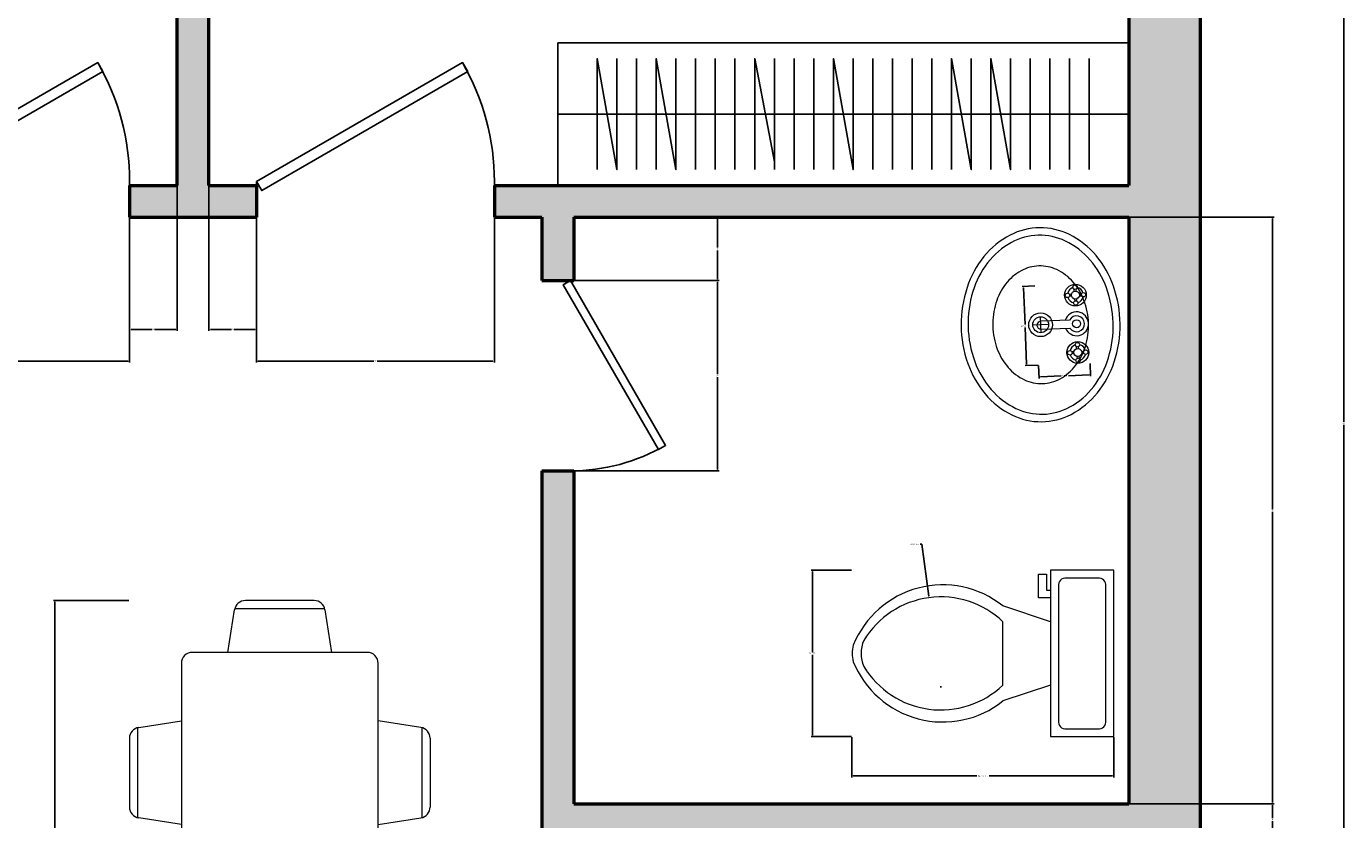
# Model space of a CAD drawing. Units: inches. Extents: x 2130 to 2425, y 2862 to 3216.
# Tile 3 of 4: x 2259 to 2425, y 2989 to 3089. Entities that reach past the tile are written whole.
import ezdxf

# ---------------------------------------------------------------- set-up
doc = ezdxf.new("R2010")
doc.units = ezdxf.units.IN
for name, color, linetype, lineweight in [('A-ANNO-DIMS', 2, 'Continuous', 18), ('A-DOOR', 3, 'Continuous', 25), ('A-FLOR-CASE', 9, 'Continuous', 25), ('A-FLOR-FIXT', 9, 'Continuous', 18), ('A-FURN', 8, 'Continuous', 18), ('A-WALL', 7, 'Continuous', 50), ('A-WALL-PATT', 18, 'Continuous', 13)]:
    doc.layers.add(name, color=color, linetype=linetype, lineweight=lineweight)
doc.styles.get("Standard").update_dxf_attribs({"font": 'arial.ttf'})
doc.dimstyles.get("Standard").update_dxf_attribs({"dimtxt": 0.18, "dimasz": 0.18, "dimexe": 0.18, "dimexo": 0.0625, "dimgap": 0.09, "dimtad": 0, "dimtih": 1, "dimtoh": 1, "dimdec": 4, "dimzin": 0, "dimdsep": 46, "dimtxsty": 'Standard', "dimcen": 0.09, "dimadec": 0, "dimazin": 0, "dimtfac": 1, "dimtdec": 4, "dimtofl": 0, "dimtmove": 0, "dimatfit": 3, "dimfxl": 1, "dimtolj": 1, "dimtzin": 0, "dimarcsym": 0})

# ---------------------------------------------------------------- blocks, each defined once
blk = doc.blocks.new('Toilet - top')
for p, q in [((9.5, -6), (9.5, -2)), ((-8, -8.5), (-8, -8)), ((-7, -8), (-7, -9.5)), ((-4, -8), (-6, -14)), ((4, -8), (6, -14)), ((-10, -8.5), (-8, -8.5)), ((-10, -9.5), (-10, -8.5)), ((-7, -9.5), (-10, -9.5)), ((4, -14), (-4, -14))]:
    blk.add_line(p, q)
blk.add_lwpolyline([(10.5, -8), (10.5, 0), (-10.5, 0), (-10.5, -8)], close=True)
for points in [[(8.5, -1), (-8.5, -1)], [(-9.5, -2), (-9.5, -6)], [(-8.5, -7), (8.5, -7)]]:
    blk.add_lwpolyline(points)
for centre, radius, start, end in [((-8.62, -1.88), 0.884, 81.8699, 188.1301), ((8.62, -1.88), 0.884, 351.8699, 98.1301), ((-8.62, -6.12), 0.884, 171.8699, 278.1301), ((8.62, -6.12), 0.884, 261.8699, 8.1301), ((3.52, -21.58), 12.17, 141.4691, 247.9714), ((4.2, -21.82), 11.33, 136.3677, 238.9468), ((-3.52, -21.58), 12.17, 292.0284, 38.5307), ((-4.2, -21.82), 11.33, 301.053, 43.6321), ((0, -27.88), 4, 245.7318, 294.2682), ((0, -29), 4, 254.8605, 285.1395)]:
    blk.add_arc(centre, radius, start, end)
blk = doc.blocks.new('Dining Set - 36 x 72 in.')
for p, q in [((-20.29, 27.5), (-7.71, 27.5)), ((7.71, 27.5), (20.29, 27.5)), ((-22.26, 25.81), (-23.48, 18)), ((-22.23, 26), (-5.76, 26)), ((-4.52, 18), (-5.74, 25.81)), ((5.74, 25.81), (4.52, 18)), ((5.77, 26), (22.24, 26)), ((23.48, 18), (22.26, 25.81)), ((34, 18), (-34, 18)), ((-36, 16), (-36, -16)), ((36, -16), (36, 16)), ((-44, 8.23), (-44, -8.24)), ((-43.81, 8.26), (-36, 9.48)), ((43.81, 8.26), (36, 9.48)), ((44, 8.23), (44, -8.24)), ((-45.5, 6.29), (-45.5, -6.29)), ((45.5, 6.29), (45.5, -6.29)), ((-36, -9.48), (-43.81, -8.26)), ((36, -9.48), (43.81, -8.26)), ((-34, -18), (34, -18)), ((-22.26, -25.81), (-23.48, -18)), ((-4.52, -18), (-5.74, -25.81)), ((5.74, -25.81), (4.52, -18)), ((23.48, -18), (22.26, -25.81)), ((-22.23, -26), (-5.76, -26)), ((5.77, -26), (22.24, -26)), ((-20.29, -27.5), (-7.71, -27.5)), ((7.71, -27.5), (20.29, -27.5))]:
    blk.add_line(p, q)
for centre, start, end in [((-20.29, 25.5), 90, 171.1198), ((-7.71, 25.5), 8.881, 90), ((7.71, 25.5), 90, 171.1198), ((20.29, 25.5), 8.881, 90), ((-34, 16), 90, 180), ((34, 16), 0, 90), ((-43.5, 6.29), 98.8806, 180), ((43.5, 6.29), 0, 81.1194), ((-43.5, -6.29), 180, 261.1194), ((43.5, -6.29), 278.8806, 0), ((-34, -16), 180, 270), ((34, -16), 270, 0), ((-20.29, -25.5), 188.8802, 270), ((-7.71, -25.5), 270, 351.1191), ((7.71, -25.5), 188.8802, 270), ((20.29, -25.5), 270, 351.1191)]:
    blk.add_arc(centre, 2, start, end)
blk = doc.blocks.new('Sink - Oval top')
for p, q in [((-1, 0), (1, 0)), ((0, 1), (0, -1))]:
    blk.add_line(p, q)
for points in [[(-12.23, 0.39, 0.117634), (-11.46, -3.36, 0.104469), (-8.88, -6.8, 0.090016), (-5.08, -9.07, 0.08192), (-0.32, -10.02, 0.08192), (4.49, -9.38, 0.090016), (8.42, -7.36, 0.104469), (11.22, -4.09, 0.117634), (12.23, -0.39, 0.117634), (11.46, 3.36, 0.104469), (8.88, 6.8, 0.090016), (5.08, 9.07, 0.08192), (0.32, 10.02, 0.08192), (-4.49, 9.38, 0.090016), (-8.42, 7.36, 0.104469), (-11.22, 4.09, 0.117634)], [(-11.29, 0.16, 0.118622), (-10.52, -3.25, 0.104678), (-8.07, -6.36, 0.089562), (-4.54, -8.37, 0.081185), (-0.13, -9.15, 0.081185), (4.3, -8.49, 0.089562), (7.89, -6.58, 0.104678), (10.42, -3.55, 0.118622), (11.29, -0.16, 0.118622), (10.52, 3.25, 0.104678), (8.07, 6.36, 0.089562), (4.54, 8.37, 0.081185), (0.13, 9.15, 0.081185), (-4.3, 8.49, 0.089562), (-7.89, 6.58, 0.104678), (-10.42, 3.55, 0.118622)], [(-7.42, 0.08, 0.118283), (-6.91, -2.17, 0.104607), (-5.29, -4.21, 0.089718), (-2.97, -5.53, 0.081436), (-0.07, -6.04, 0.081436), (2.84, -5.59, 0.089718), (5.2, -4.33, 0.104607), (6.86, -2.32, 0.118283), (7.42, -0.08, 0.118283), (6.91, 2.17, 0.104607), (5.29, 4.21, 0.089718), (2.97, 5.53, 0.081436), (0.07, 6.04, 0.081436), (-2.84, 5.59, 0.089718), (-5.2, 4.33, 0.104607), (-6.86, 2.32, 0.118283)]]:
    blk.add_lwpolyline(points, format="xyb", close=True)
for radius in [1.5, 1]:
    blk.add_circle((0, 0), radius)
blk = doc.blocks.new('Faucet - Bathroom top')
for p, q in [((-4.107, 0.125), (-4.375, 0.125)), ((-3.75, 0.4788), (-3.75, 0.75)), ((-3.5, 0.482), (-3.5, 0.75)), ((-3.1461, 0.125), (-2.875, 0.125)), ((3.143, 0.125), (2.875, 0.125)), ((3.5, 0.4788), (3.5, 0.75)), ((3.75, 0.482), (3.75, 0.75)), ((4.1039, 0.125), (4.375, 0.125)), ((-4.1039, -0.125), (-4.375, -0.125)), ((-3.75, -0.4821), (-3.75, -0.75)), ((-3.5, -0.4789), (-3.5, -0.75)), ((-3.143, -0.125), (-2.875, -0.125)), ((-0.5, -0.8639), (-0.5, -4.5)), ((0.5, -4.5), (0.5, -0.8631)), ((3.1461, -0.125), (2.875, -0.125)), ((3.5, -0.4821), (3.5, -0.75)), ((3.75, -0.4789), (3.75, -0.75)), ((4.107, -0.125), (4.375, -0.125))]:
    blk.add_line(p, q)
for centre, radius in [((-3.625, 0), 1.375), ((-4.625, 0), 0.2795), ((-3.625, 0), 0.5), ((-3.625, 1), 0.2795), ((-2.625, 0), 0.2795), ((0, 0), 0.5), ((3.625, 0), 1.375), ((2.625, 0), 0.2795), ((3.625, 0), 0.5), ((3.625, 1), 0.2795), ((4.625, 0), 0.2795), ((-3.625, -1), 0.2795), ((3.625, -1), 0.2795)]:
    blk.add_circle(centre, radius)
for centre, radius, start, end in [((-3.625, 0), 1, 105.2407, 164.2093), ((-3.625, 0), 1, 16.44125, 74.07887), ((0, 0), 1.5, 289.6514, 250.3603), ((0, 0), 1, 300.3431, 239.7554), ((3.625, 0), 1, 106.12, 164.0884), ((3.625, 0), 1, 16.23422, 73.90469), ((-3.625, 0), 1, 196.2342, 253.9047), ((-3.625, 0), 1, 286.12, 344.0884), ((3.625, 0), 1, 196.4413, 254.0789), ((3.625, 0), 1, 285.2407, 344.2093), ((0, -4.5), 0.5, 180, 0)]:
    blk.add_arc(centre, radius, start, end)
blk = doc.blocks.new('*U10')
for p, q in [((0, 0), (0, -6)), ((40, 0), (40, -6))]:
    blk.add_line(p, q)
blk.add_lwpolyline([(0, 0), (34.64, 20), (35.52, 18.48), (0.87, -1.52)], close=True)
blk.add_arc((0, 0), 40, 0, 30)
blk = doc.blocks.new('WARDROBE-72X18IN')
for p, q in [((0, 0), (0, 72)), ((0, 72), (18, 72)), ((9, 72), (9, 0)), ((18, 72), (18, 0)), ((2, 62.07), (16, 62.07)), ((2, 54.62), (16, 54.62)), ((2, 52.14), (16, 52.14)), ((2, 49.66), (16, 49.66)), ((2, 44.69), (16, 44.69)), ((2, 42.21), (16, 42.21)), ((2, 39.72), (16, 39.72)), ((2, 32.28), (16, 32.28)), ((2, 29.79), (16, 29.79)), ((2, 27.31), (16, 27.31)), ((2, 24.83), (16, 24.83)), ((2, 12.41), (16, 12.41)), ((2, 9.93), (16, 9.93)), ((2, 7.45), (16, 7.45)), ((2, 4.97), (16, 4.97)), ((18, 0), (0, 0))]:
    blk.add_line(p, q)
for points in [[(2, 67.03), (16, 67.03), (2, 64.55), (16, 64.55)], [(2, 59.59), (16, 59.59), (2, 57.1), (16, 57.1)], [(2, 47.17), (16, 47.17), (2.98, 44.69)], [(2, 37.24), (16, 37.24), (2, 34.76), (16, 34.76)], [(2, 22.35), (16, 22.35), (2, 19.86), (16, 19.86)], [(2, 17.38), (16, 17.38), (2, 14.9), (16, 14.9)]]:
    blk.add_lwpolyline(points)
blk.add_lwpolyline([(0, 0), (18, 0)], close=True)
blk = doc.blocks.new('*D21')
at = {"layer": 'A-ANNO-DIMS', "color": 0, "lineweight": -2, "transparency": 16777216}
for p, q in [((2362.63, 2999.36), (2362.63, 2994.28)), ((2395.68, 2999.36), (2395.68, 2994.28)), ((2362.81, 2994.46), (2378.38, 2994.46)), ((2395.5, 2994.46), (2379.93, 2994.46))]:
    blk.add_line(p, q, dxfattribs=at)
at = {"layer": 'A-ANNO-DIMS', "color": 0, "transparency": 16777216}
for points in [[(2362.81, 2994.49), (2362.81, 2994.43), (2362.63, 2994.46)], [(2395.5, 2994.49), (2395.5, 2994.43), (2395.68, 2994.46)]]:
    blk.add_solid(points, dxfattribs=at)
at = {"layer": 'Defpoints', "color": 0, "transparency": 16777216}
for p in [(2362.63, 2999.42), (2395.68, 2999.42), (2395.68, 2994.46)]:
    blk.add_point(p, dxfattribs=at)
at = {"layer": 'A-ANNO-DIMS', "color": 0, "transparency": 16777216, "insert": (2379.15, 2994.46), "char_height": 0.18, "attachment_point": 5}
blk.add_mtext('\\A1;WC 33 TYP.', dxfattribs=at)
blk = doc.blocks.new('*D22')
at = {"layer": 'A-ANNO-DIMS', "color": 0, "lineweight": -2, "transparency": 16777216}
for p, q in [((2362.57, 3020.42), (2357.49, 3020.42)), ((2357.67, 3020.24), (2357.67, 3010.1)), ((2357.67, 2999.6), (2357.67, 3009.74)), ((2362.57, 2999.42), (2357.49, 2999.42))]:
    blk.add_line(p, q, dxfattribs=at)
at = {"layer": 'A-ANNO-DIMS', "color": 0, "transparency": 16777216}
for points in [[(2357.64, 3020.24), (2357.7, 3020.24), (2357.67, 3020.42)], [(2357.64, 2999.6), (2357.7, 2999.6), (2357.67, 2999.42)]]:
    blk.add_solid(points, dxfattribs=at)
at = {"layer": 'Defpoints', "color": 0, "transparency": 16777216}
for p in [(2362.63, 3020.42), (2357.67, 2999.42), (2362.63, 2999.42)]:
    blk.add_point(p, dxfattribs=at)
at = {"layer": 'A-ANNO-DIMS', "color": 0, "transparency": 16777216, "insert": (2357.67, 3009.92), "char_height": 0.18, "attachment_point": 5}
blk.add_mtext('\\A1;21 TYP.', dxfattribs=at)
blk = doc.blocks.new('*D25')
at = {"layer": 'A-ANNO-DIMS', "color": 0, "lineweight": -2, "transparency": 16777216}
for p, q in [((2385.71, 3056.29), (2384.1, 3056.22)), ((2384.28, 3056.05), (2384.48, 3051.42)), ((2384.68, 3046.42), (2384.49, 3051.05)), ((2386.13, 3046.3), (2384.51, 3046.23))]:
    blk.add_line(p, q, dxfattribs=at)
at = {"layer": 'A-ANNO-DIMS', "color": 0, "transparency": 16777216}
for points in [[(2384.31, 3056.05), (2384.25, 3056.05), (2384.28, 3056.23)], [(2384.71, 3046.42), (2384.65, 3046.42), (2384.69, 3046.24)]]:
    blk.add_solid(points, dxfattribs=at)
at = {"layer": 'Defpoints', "color": 0, "transparency": 16777216}
for p in [(2385.78, 3056.29), (2384.69, 3046.24), (2386.19, 3046.3)]:
    blk.add_point(p, dxfattribs=at)
at = {"layer": 'A-ANNO-DIMS', "color": 0, "transparency": 16777216, "insert": (2384.48, 3051.24), "char_height": 0.18, "attachment_point": 5}
blk.add_mtext('\\A1;TAP 10 TYP.', dxfattribs=at)
blk = doc.blocks.new('*D26')
at = {"layer": 'A-ANNO-DIMS', "color": 0, "lineweight": -2, "transparency": 16777216}
for p, q in [((2392.69, 3046.51), (2392.75, 3044.89)), ((2386.19, 3046.24), (2386.26, 3044.62)), ((2386.43, 3044.81), (2389.04, 3044.92)), ((2392.57, 3045.07), (2389.96, 3044.96))]:
    blk.add_line(p, q, dxfattribs=at)
at = {"layer": 'A-ANNO-DIMS', "color": 0, "transparency": 16777216}
for points in [[(2386.43, 3044.84), (2386.43, 3044.78), (2386.25, 3044.8)], [(2392.57, 3045.1), (2392.57, 3045.04), (2392.75, 3045.07)]]:
    blk.add_solid(points, dxfattribs=at)
at = {"layer": 'Defpoints', "color": 0, "transparency": 16777216}
for p in [(2392.68, 3046.57), (2386.19, 3046.3), (2392.75, 3045.07)]:
    blk.add_point(p, dxfattribs=at)
at = {"layer": 'A-ANNO-DIMS', "color": 0, "transparency": 16777216, "insert": (2389.5, 3044.94), "char_height": 0.18, "attachment_point": 5}
blk.add_mtext('\\A1;7 TYP.', dxfattribs=at)
blk = doc.blocks.new('*D29')
at = {"layer": 'A-ANNO-DIMS', "color": 0, "lineweight": -2, "transparency": 16777216}
for p, q in [((2271.46, 3016.6), (2261.94, 3016.6)), ((2262.12, 3016.42), (2262.12, 2985.41)), ((2262.12, 2954.04), (2262.12, 2985.05)), ((2271.46, 2953.86), (2261.94, 2953.86))]:
    blk.add_line(p, q, dxfattribs=at)
at = {"layer": 'A-ANNO-DIMS', "color": 0, "transparency": 16777216}
for points in [[(2262.09, 3016.42), (2262.15, 3016.42), (2262.12, 3016.6)], [(2262.09, 2954.04), (2262.15, 2954.04), (2262.12, 2953.86)]]:
    blk.add_solid(points, dxfattribs=at)
at = {"layer": 'Defpoints', "color": 0, "transparency": 16777216}
for p in [(2271.53, 3016.6), (2262.12, 2953.86), (2271.53, 2953.86)]:
    blk.add_point(p, dxfattribs=at)
at = {"layer": 'A-ANNO-DIMS', "color": 0, "transparency": 16777216, "insert": (2262.12, 2985.23), "char_height": 0.18, "attachment_point": 5}
blk.add_mtext('\\A1;DINING SET 63', dxfattribs=at)
blk = doc.blocks.new('*D36')
at = {"layer": 'A-ANNO-DIMS', "color": 0, "lineweight": -2, "transparency": 16777216}
for p, q in [((2406.61, 3197.95), (2424.88, 3197.95)), ((2424.7, 3197.77), (2424.7, 3039.14)), ((2424.7, 2880.13), (2424.7, 3038.77)), ((2406.61, 2879.95), (2424.88, 2879.95))]:
    blk.add_line(p, q, dxfattribs=at)
at = {"layer": 'A-ANNO-DIMS', "color": 0, "transparency": 16777216}
for points in [[(2424.67, 3197.77), (2424.73, 3197.77), (2424.7, 3197.95)], [(2424.67, 2880.13), (2424.73, 2880.13), (2424.7, 2879.95)]]:
    blk.add_solid(points, dxfattribs=at)
at = {"layer": 'Defpoints', "color": 0, "transparency": 16777216}
for p in [(2406.55, 3197.95), (2424.7, 3197.95), (2406.55, 2879.95)]:
    blk.add_point(p, dxfattribs=at)
at = {"layer": 'A-ANNO-DIMS', "color": 0, "transparency": 16777216, "insert": (2424.7, 3038.95), "char_height": 0.18, "attachment_point": 5}
blk.add_mtext('\\A1;318', dxfattribs=at)
blk = doc.blocks.new('*D54')
at = {"layer": 'A-ANNO-DIMS', "color": 0, "lineweight": -2, "transparency": 16777216}
for p, q in [((2397.612727, 3064.954394), (2415.880227, 3064.954394)), ((2415.700227, 3064.774394), (2415.700227, 3028.134394)), ((2415.700227, 2991.134394), (2415.700227, 3027.774394)), ((2397.612727, 2990.954394), (2415.880227, 2990.954394))]:
    blk.add_line(p, q, dxfattribs=at)
at = {"layer": 'A-ANNO-DIMS', "color": 0, "transparency": 16777216}
for points in [[(2415.670227, 3064.774394), (2415.730227, 3064.774394), (2415.700227, 3064.954394)], [(2415.670227, 2991.134394), (2415.730227, 2991.134394), (2415.700227, 2990.954394)]]:
    blk.add_solid(points, dxfattribs=at)
at = {"layer": 'Defpoints', "color": 0, "transparency": 16777216}
for p in [(2397.550227, 3064.954394), (2397.550227, 2990.954394), (2415.700227, 2990.954394)]:
    blk.add_point(p, dxfattribs=at)
at = {"layer": 'A-ANNO-DIMS', "color": 0, "transparency": 16777216, "insert": (2415.700227, 3027.954394), "char_height": 0.18, "attachment_point": 5}
blk.add_mtext('\\A1;74', dxfattribs=at)
blk = doc.blocks.new('*D55')
at = {"layer": 'A-ANNO-DIMS', "color": 0, "lineweight": -2, "transparency": 16777216}
for p, q in [((2397.612727, 2990.954394), (2415.880227, 2990.954394)), ((2415.700227, 2990.774394), (2415.700227, 2989.134394)), ((2415.700227, 2987.134394), (2415.700227, 2988.774394)), ((2397.612727, 2986.954394), (2415.880227, 2986.954394))]:
    blk.add_line(p, q, dxfattribs=at)
at = {"layer": 'A-ANNO-DIMS', "color": 0, "transparency": 16777216}
for points in [[(2415.670227, 2990.774394), (2415.730227, 2990.774394), (2415.700227, 2990.954394)], [(2415.670227, 2987.134394), (2415.730227, 2987.134394), (2415.700227, 2986.954394)]]:
    blk.add_solid(points, dxfattribs=at)
at = {"layer": 'Defpoints', "color": 0, "transparency": 16777216}
for p in [(2397.550227, 2990.954394), (2397.550227, 2986.954394), (2415.700227, 2986.954394)]:
    blk.add_point(p, dxfattribs=at)
at = {"layer": 'A-ANNO-DIMS', "color": 0, "transparency": 16777216, "insert": (2415.700227, 2988.954394), "char_height": 0.18, "attachment_point": 5}
blk.add_mtext('\\A1;4', dxfattribs=at)
blk = doc.blocks.new('*D57')
at = {"layer": 'A-ANNO-DIMS', "color": 0, "lineweight": -2, "transparency": 16777216}
for p, q in [((2241.55, 3064.89), (2241.55, 3046.62)), ((2271.55, 3064.89), (2271.55, 3046.62)), ((2241.73, 3046.8), (2256.33, 3046.8)), ((2271.37, 3046.8), (2256.77, 3046.8))]:
    blk.add_line(p, q, dxfattribs=at)
at = {"layer": 'A-ANNO-DIMS', "color": 0, "transparency": 16777216}
for points in [[(2241.73, 3046.83), (2241.73, 3046.77), (2241.55, 3046.8)], [(2271.37, 3046.83), (2271.37, 3046.77), (2271.55, 3046.8)]]:
    blk.add_solid(points, dxfattribs=at)
at = {"layer": 'Defpoints', "color": 0, "transparency": 16777216}
for p in [(2241.55, 3064.95), (2271.55, 3064.95), (2241.55, 3046.8)]:
    blk.add_point(p, dxfattribs=at)
at = {"layer": 'A-ANNO-DIMS', "color": 0, "transparency": 16777216, "insert": (2256.55, 3046.8), "char_height": 0.18, "attachment_point": 5}
blk.add_mtext('\\A1;30', dxfattribs=at)
blk = doc.blocks.new('*D58')
at = {"layer": 'A-ANNO-DIMS', "color": 0, "lineweight": -2, "transparency": 16777216}
for p, q in [((2271.55, 3068.89), (2271.55, 3050.62)), ((2277.55, 3068.89), (2277.55, 3050.62)), ((2271.73, 3050.8), (2274.4, 3050.8)), ((2277.37, 3050.8), (2274.7, 3050.8))]:
    blk.add_line(p, q, dxfattribs=at)
at = {"layer": 'A-ANNO-DIMS', "color": 0, "transparency": 16777216}
for points in [[(2271.73, 3050.83), (2271.73, 3050.77), (2271.55, 3050.8)], [(2277.37, 3050.83), (2277.37, 3050.77), (2277.55, 3050.8)]]:
    blk.add_solid(points, dxfattribs=at)
at = {"layer": 'Defpoints', "color": 0, "transparency": 16777216}
for p in [(2271.55, 3068.95), (2277.55, 3068.95), (2271.55, 3050.8)]:
    blk.add_point(p, dxfattribs=at)
at = {"layer": 'A-ANNO-DIMS', "color": 0, "transparency": 16777216, "insert": (2274.55, 3050.8), "char_height": 0.18, "attachment_point": 5}
blk.add_mtext('\\A1;6', dxfattribs=at)
blk = doc.blocks.new('*D59')
at = {"layer": 'A-ANNO-DIMS', "color": 0, "lineweight": -2, "transparency": 16777216}
for p, q in [((2281.55, 3068.89), (2281.55, 3050.62)), ((2287.55, 3068.89), (2287.55, 3050.62)), ((2281.73, 3050.8), (2284.4, 3050.8)), ((2287.37, 3050.8), (2284.7, 3050.8))]:
    blk.add_line(p, q, dxfattribs=at)
at = {"layer": 'A-ANNO-DIMS', "color": 0, "transparency": 16777216}
for points in [[(2281.73, 3050.83), (2281.73, 3050.77), (2281.55, 3050.8)], [(2287.37, 3050.83), (2287.37, 3050.77), (2287.55, 3050.8)]]:
    blk.add_solid(points, dxfattribs=at)
at = {"layer": 'Defpoints', "color": 0, "transparency": 16777216}
for p in [(2281.55, 3068.95), (2287.55, 3068.95), (2281.55, 3050.8)]:
    blk.add_point(p, dxfattribs=at)
at = {"layer": 'A-ANNO-DIMS', "color": 0, "transparency": 16777216, "insert": (2284.55, 3050.8), "char_height": 0.18, "attachment_point": 5}
blk.add_mtext('\\A1;6', dxfattribs=at)
blk = doc.blocks.new('*D60')
at = {"layer": 'A-ANNO-DIMS', "color": 0, "lineweight": -2, "transparency": 16777216}
for p, q in [((2287.55, 3064.89), (2287.55, 3046.62)), ((2317.55, 3064.89), (2317.55, 3046.62)), ((2287.73, 3046.8), (2302.33, 3046.8)), ((2317.37, 3046.8), (2302.77, 3046.8))]:
    blk.add_line(p, q, dxfattribs=at)
at = {"layer": 'A-ANNO-DIMS', "color": 0, "transparency": 16777216}
for points in [[(2287.73, 3046.83), (2287.73, 3046.77), (2287.55, 3046.8)], [(2317.37, 3046.83), (2317.37, 3046.77), (2317.55, 3046.8)]]:
    blk.add_solid(points, dxfattribs=at)
at = {"layer": 'Defpoints', "color": 0, "transparency": 16777216}
for p in [(2287.55, 3064.95), (2317.55, 3064.95), (2287.55, 3046.8)]:
    blk.add_point(p, dxfattribs=at)
at = {"layer": 'A-ANNO-DIMS', "color": 0, "transparency": 16777216, "insert": (2302.55, 3046.8), "char_height": 0.18, "attachment_point": 5}
blk.add_mtext('\\A1;30', dxfattribs=at)
blk = doc.blocks.new('*D63')
at = {"layer": 'A-ANNO-DIMS', "color": 0, "lineweight": -2, "transparency": 16777216}
for p, q in [((2327.61, 3056.95), (2345.88, 3056.95)), ((2345.7, 3056.77), (2345.7, 3045.13)), ((2345.7, 3033.13), (2345.7, 3044.77)), ((2327.61, 3032.95), (2345.88, 3032.95))]:
    blk.add_line(p, q, dxfattribs=at)
at = {"layer": 'A-ANNO-DIMS', "color": 0, "transparency": 16777216}
for points in [[(2345.67, 3056.77), (2345.73, 3056.77), (2345.7, 3056.95)], [(2345.67, 3033.13), (2345.73, 3033.13), (2345.7, 3032.95)]]:
    blk.add_solid(points, dxfattribs=at)
at = {"layer": 'Defpoints', "color": 0, "transparency": 16777216}
for p in [(2327.55, 3056.95), (2327.55, 3032.95), (2345.7, 3032.95)]:
    blk.add_point(p, dxfattribs=at)
at = {"layer": 'A-ANNO-DIMS', "color": 0, "transparency": 16777216, "insert": (2345.7, 3044.95), "char_height": 0.18, "attachment_point": 5}
blk.add_mtext('\\A1;24', dxfattribs=at)
blk = doc.blocks.new('*D64')
at = {"layer": 'A-ANNO-DIMS', "color": 0, "lineweight": -2, "transparency": 16777216}
for p, q in [((2327.61, 3064.95), (2345.88, 3064.95)), ((2345.7, 3064.77), (2345.7, 3061.14)), ((2345.7, 3057.13), (2345.7, 3060.77)), ((2327.61, 3056.95), (2345.88, 3056.95))]:
    blk.add_line(p, q, dxfattribs=at)
at = {"layer": 'A-ANNO-DIMS', "color": 0, "transparency": 16777216}
for points in [[(2345.67, 3064.77), (2345.73, 3064.77), (2345.7, 3064.95)], [(2345.67, 3057.13), (2345.73, 3057.13), (2345.7, 3056.95)]]:
    blk.add_solid(points, dxfattribs=at)
at = {"layer": 'Defpoints', "color": 0, "transparency": 16777216}
for p in [(2327.55, 3064.95), (2327.55, 3056.95), (2345.7, 3056.95)]:
    blk.add_point(p, dxfattribs=at)
at = {"layer": 'A-ANNO-DIMS', "color": 0, "transparency": 16777216, "insert": (2345.7, 3060.95), "char_height": 0.18, "attachment_point": 5}
blk.add_mtext('\\A1;8', dxfattribs=at)
blk = doc.blocks.new('*D75')
at = {"layer": 'A-ANNO-DIMS', "color": 0, "lineweight": -2, "transparency": 16777216}
for p, q in [((2371.26, 3023.69), (2371.44, 3023.69)), ((2371.44, 3023.69), (2372.33, 3017.13)), ((2373.77, 3005.72), (2373.95, 3005.72)), ((2373.86, 3005.63), (2373.86, 3005.81))]:
    blk.add_line(p, q, dxfattribs=at)
at = {"layer": 'A-ANNO-DIMS', "color": 0, "transparency": 16777216}
blk.add_solid([(2372.36, 3017.13), (2372.3, 3017.12), (2372.35, 3016.95)], dxfattribs=at)
at = {"layer": 'Defpoints', "color": 0, "transparency": 16777216}
for p in [(2372.35, 3016.95), (2373.86, 3005.72)]:
    blk.add_point(p, dxfattribs=at)
at = {"layer": 'A-ANNO-DIMS', "color": 0, "transparency": 16777216, "insert": (2370.59, 3023.69), "char_height": 0.18, "attachment_point": 5}
blk.add_mtext('\\A1;4X R11.33', dxfattribs=at)

msp = doc.modelspace()

# ---------------------------------------------------------------- hatches: boundary and pattern name
at = {"layer": 'A-WALL-PATT'}
h = msp.add_hatch(color=256, dxfattribs=at)
h.dxf.hatch_style = 1
h.paths.add_polyline_path([(2319.6433, 3197.9544), (2234.3228, 3197.9544), (2234.3228, 3188.9544), (2277.5502, 3188.9544), (2277.5502, 3116.9544), (2277.5502, 3068.9544), (2271.5502, 3068.9544), (2271.5502, 3064.9544), (2281.5502, 3064.9544), (2287.5502, 3064.9544), (2287.5502, 3068.9544), (2281.5502, 3068.9544), (2281.5502, 3188.9544), (2319.6433, 3188.9544)])
h = msp.add_hatch(color=256, dxfattribs=at)
h.dxf.hatch_style = 1
h.paths.add_polyline_path([(2406.5502, 3197.9544), (2367.6433, 3197.9544), (2367.6433, 3188.9544), (2397.5502, 3188.9544), (2397.5502, 3068.9544), (2325.5502, 3068.9544), (2317.5502, 3068.9544), (2317.5502, 3064.9544), (2323.5502, 3064.9544), (2323.5502, 3056.9544), (2327.5502, 3056.9544), (2327.5502, 3064.9544), (2397.5502, 3064.9544), (2397.5502, 2990.9544), (2327.5502, 2990.9544), (2327.5502, 3032.9544), (2323.5502, 3032.9544), (2323.5502, 2986.9544), (2323.5502, 2961.9544), (2327.5502, 2961.9544), (2327.5502, 2986.9544), (2397.5502, 2986.9544), (2397.5502, 2966.8556), (2406.5502, 2966.8556)])

# ---------------------------------------------------------------- linework, layer by layer
at = {"layer": 'A-WALL'}
for p, q in [((2277.5502, 3068.9544), (2277.5502, 3188.9544)), ((2281.5502, 3068.9544), (2281.5502, 3188.9544)), ((2397.5502, 3188.9544), (2397.5502, 3068.9544)), ((2271.5502, 3068.9544), (2271.5502, 3064.9544)), ((2271.5502, 3068.9544), (2277.5502, 3068.9544)), ((2281.5502, 3068.9544), (2287.5502, 3068.9544)), ((2287.5502, 3068.9544), (2287.5502, 3064.9544)), ((2317.5502, 3068.9544), (2317.5502, 3064.9544)), ((2317.5502, 3068.9544), (2397.5502, 3068.9544)), ((2271.5502, 3064.9544), (2281.5502, 3064.9544)), ((2281.5502, 3064.9544), (2287.5502, 3064.9544)), ((2317.5502, 3064.9544), (2323.5502, 3064.9544)), ((2323.5502, 3064.9544), (2323.5502, 3056.9544)), ((2327.5502, 3064.9544), (2327.5502, 3056.9544)), ((2327.5502, 3064.9544), (2397.5502, 3064.9544)), ((2397.5502, 3064.9544), (2397.5502, 2990.9544)), ((2323.5502, 3056.9544), (2327.5502, 3056.9544)), ((2323.5502, 3032.9544), (2327.5502, 3032.9544)), ((2323.5502, 3032.9544), (2323.5502, 2986.9544)), ((2327.5502, 3032.9544), (2327.5502, 2990.9544)), ((2327.5502, 2990.9544), (2397.5502, 2990.9544))]:
    msp.add_line(p, q, dxfattribs=at)
msp.add_lwpolyline([(2163.5502, 2879.9544), (2148.5502, 2879.9544), (2148.5502, 3197.9544), (2406.5502, 3197.9544), (2406.5502, 2879.9544), (2211.5502, 2879.9544)], dxfattribs=at)

# ---------------------------------------------------------------- block references
at = {"layer": 'A-DOOR', "xscale": 0.75, "yscale": 0.75, "zscale": 0.75}
for p in [(2241.5502, 3069.4544), (2287.5502, 3069.4544)]:
    msp.add_blockref('*U10', p, dxfattribs=at)
at = {"layer": 'A-DOOR', "xscale": 0.6, "yscale": 0.6, "zscale": 0.6, "rotation": 270}
msp.add_blockref('*U10', (2327.1502, 3056.9544), dxfattribs=at)
at = {"layer": 'A-FLOR-CASE', "rotation": 90.00000000000817}
msp.add_blockref('WARDROBE-72X18IN', (2397.5506, 3068.9542), dxfattribs=at)
at = {"layer": 'A-FLOR-FIXT'}
for name, p, rotation in [('Sink - Oval top', (2386.4425, 3051.3856), 272.3762008697443), ('Faucet - Bathroom top', (2390.9782, 3051.5061), 272.3762008697443), ('Toilet - top', (2395.6767, 3009.9202), 269.9999999999966)]:
    msp.add_blockref(name, p, dxfattribs=dict(at, rotation=rotation))
at = {"layer": 'A-FURN', "xscale": 0.6894662824826121, "yscale": 0.6894662824826121, "zscale": 0.6894662824826121, "rotation": 270}
msp.add_blockref('Dining Set - 36 x 72 in.', (2290.487, 2985.2285), dxfattribs=at)

# ---------------------------------------------------------------- dimensions: what is measured, and where the dimension line sits
at = {"layer": 'A-ANNO-DIMS'}
for base, p1, p2, angle, picture, middle in [((2424.7002, 3197.9544), (2406.5502, 2879.9544), (2406.5502, 3197.9544), 90, '*D36', (2424.7002, 3038.9544)), ((2271.5502, 3050.8044), (2277.5502, 3068.9544), (2271.5502, 3068.9544), 180, '*D58', (2274.5502, 3050.8044)), ((2281.5502, 3050.8044), (2287.5502, 3068.9544), (2281.5502, 3068.9544), 180, '*D59', (2284.5502, 3050.8044)), ((2241.5502, 3046.8044), (2271.5502, 3064.9544), (2241.5502, 3064.9544), 180, '*D57', (2256.5502, 3046.8044)), ((2287.5502, 3046.8044), (2317.5502, 3064.9544), (2287.5502, 3064.9544), 180, '*D60', (2302.5502, 3046.8044)), ((2345.7002, 3056.9544), (2327.5502, 3064.9544), (2327.5502, 3056.9544), 270, '*D64', (2345.7002, 3060.9544)), ((2415.7002, 2990.9544), (2397.5502, 3064.9544), (2397.5502, 2990.9544), 270, '*D54', (2415.7002, 3027.9544)), ((2345.7002, 3032.9544), (2327.5502, 3056.9544), (2327.5502, 3032.9544), 270, '*D63', (2345.7002, 3044.9544)), ((2415.7002, 2986.9544), (2397.5502, 2990.9544), (2397.5502, 2986.9544), 270, '*D55', (2415.7002, 2988.9544))]:
    dim = msp.add_linear_dim(base=base, p1=p1, p2=p2, angle=angle, dimstyle='Standard', override={"dimdec": 0, "dimlfac": 1, "dimrnd": 0, "dimzin": 0, "dimdsep": 46, "dimlunit": 2}, dxfattribs=at)
    dim.commit()
    dim.dimension.update_dxf_attribs({"geometry": picture, "text_midpoint": middle})
for base, p1, p2, angle, text, picture, middle in [((2384.6911, 3046.2409), (2385.7752, 3056.2945), (2386.1898, 3046.3031), 272.376201, 'TAP <> TYP.', '*D25', (2384.4838, 3051.2366)), ((2392.7464, 3045.0739), (2386.1898, 3046.3031), (2392.6843, 3046.5726), 2.376201, '<> TYP.', '*D26', (2389.4992, 3044.9392)), ((2357.6735, 2999.4202), (2362.6305, 3020.4202), (2362.6305, 2999.4202), 270, '<> TYP.', '*D22', (2357.6735, 3009.9202)), ((2262.1154, 2953.8578), (2271.5266, 3016.5993), (2271.5266, 2953.8578), 270, 'DINING SET <>', '*D29', (2262.1154, 2985.2285))]:
    dim = msp.add_linear_dim(base=base, p1=p1, p2=p2, angle=angle, text=text, dimstyle='Standard', override={"dimdec": 0, "dimlfac": 1, "dimrnd": 0, "dimzin": 0, "dimdsep": 46, "dimlunit": 2}, dxfattribs=at)
    dim.commit()
    dim.dimension.update_dxf_attribs({"geometry": picture, "text_midpoint": middle})
dim = msp.add_radius_dim(center=(2373.8593, 3005.7202), mpoint=(2372.3499, 3016.9484), text='4X <>', dimstyle='Standard', override={"dimdec": 2, "dimlfac": 1, "dimrnd": 0, "dimzin": 0, "dimdsep": 46, "dimlunit": 2}, dxfattribs=at)
dim.commit()
dim.dimension.update_dxf_attribs({"geometry": '*D75', "text_midpoint": (2370.5875, 3023.6853), "dimtype": 164})
dim = msp.add_linear_dim(base=(2395.6767, 2994.4632), p1=(2362.6305, 2999.4202), p2=(2395.6767, 2999.4202), text='WC <> TYP.', dimstyle='Standard', override={"dimdec": 0, "dimlfac": 1, "dimrnd": 0, "dimzin": 0, "dimdsep": 46, "dimlunit": 2}, dxfattribs=at)
dim.commit()
dim.dimension.update_dxf_attribs({"geometry": '*D21', "text_midpoint": (2379.1536, 2994.4632)})

doc.saveas('drawing.dxf')
